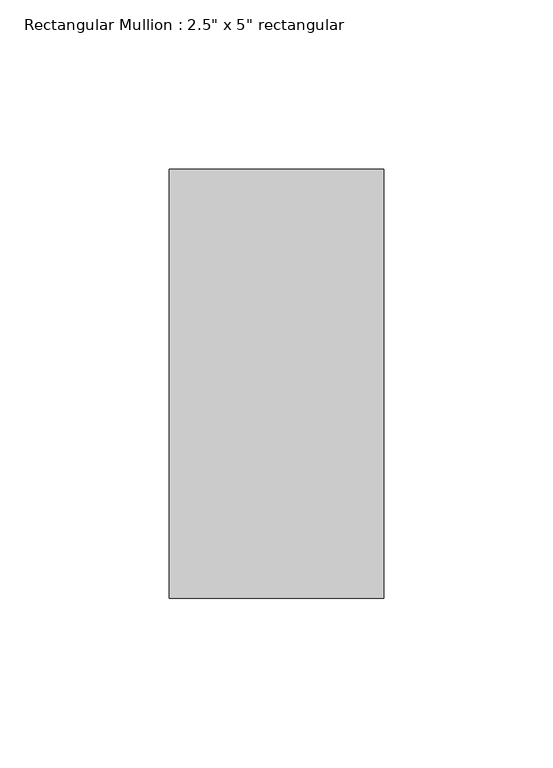
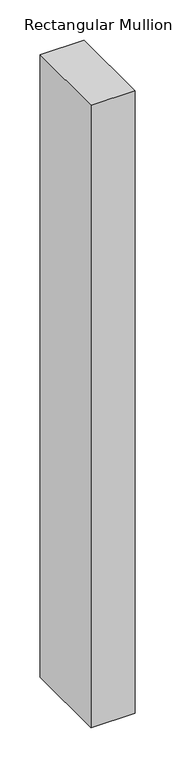
"""IFC4 building model written with IfcOpenShell, lengths in millimetres: member geometry."""

from ifc_helpers import new_model, si_unit, frame, origin, place, context, project, spatial, polyline, outline, extrude, source, transform, mapped, element, save


def member_cc8ff548(model_context):
    return source(origin(), model_context, "Body", "SweptSolid", [
        extrude(outline(polyline([(0.0, 63.5), (0.0, -63.5), (-63.5, -63.5), (-63.5, 63.5), (0.0, 63.5)])), frame((0.0, 0.0, -946.15), z_axis=(0.0, 0.0, 1.0), x_axis=(1.0, 0.0, 0.0)), (0.0, 0.0, 1.0), 946.15),
    ])


if __name__ == "__main__":
    model = new_model("IFC4")
    model_context = context("Model", 3, world=origin())
    ifc_project = project(units=[si_unit("LENGTHUNIT", "METRE", prefix="MILLI")], contexts=[model_context])
    site = spatial("IfcSite", under=ifc_project)
    building = spatial("IfcBuilding", under=site)
    placement = place(None, origin())
    member_shape = member_cc8ff548(model_context)
    element("IfcMember", 1, ObjectType="Rectangular Mullion : 2.5\" x 5\" rectangular", at=placement, inside=building, context=model_context, shape_type="MappedRepresentation", body=[
        mapped(member_shape, transform((0.0, 0.0, 0.0), x_axis=(1.0, 0.0, 0.0), y_axis=(0.0, 1.0, 0.0), z_axis=(0.0, 0.0, 1.0))),
    ])
    save(model, "model.ifc")

# Revit data of these elements
# Type "Rectangular Mullion : 2.5\" x 5\" rectangular"
#   built-in parameter 1007304 = 0.416667 (stored number, unit not read)
#   built-in parameter 1007301 = 0.104167 (stored number, unit not read)
#   built-in parameter 1007300 = 0.104167 (stored number, unit not read)
# Element 1 (IfcMember, "Rectangular Mullion : 2.5\" x 5\" rectangular")
#   Materials on its faces: "Aluminum"
# Materials
#   "Aluminum": class "Metal", colour RGB 247 247 247, transparency 0, Description = "Aluminum 6061", Cost = 0
